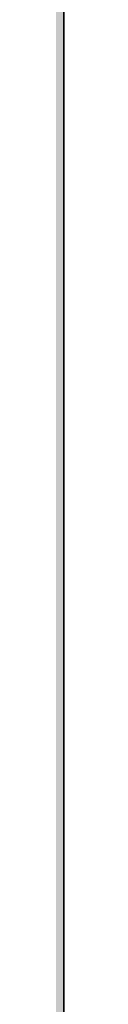
# Model space of a CAD drawing. Units: inches. Extents: x 2091 to 2899, y 967 to 2217.
# Tile 71 of 256: x 2212.144 to 2212.144, y 1102.499 to 1105.165. Entities that reach past the tile are written whole.
import ezdxf

# ---------------------------------------------------------------- set-up
doc = ezdxf.new("R2010")
doc.units = ezdxf.units.IN
doc.layers.add('A-WALL', color=7, linetype='Continuous', lineweight=35)
doc.layers.add('A-WALL-PATT', color=141, linetype='Continuous', lineweight=13, true_color=0xadddf7)

msp = doc.modelspace()

# ---------------------------------------------------------------- hatches: boundary and pattern name
at = {"layer": 'A-WALL-PATT'}
h = msp.add_hatch(color=256, dxfattribs=at)
h.dxf.hatch_style = 1
h.paths.add_polyline_path([(2212.1436, 1941.4191), (2387.6436, 1941.4191), (2387.6436, 1824.4191), (2392.1436, 1824.4191), (2392.1436, 1941.4191), (2609.6436, 1941.4191), (2609.6436, 1825.9191), (2614.1436, 1825.9191), (2614.1436, 1941.4191), (2794.1436, 1941.4191), (2794.1436, 1928.7622), (2803.1436, 1928.7622), (2803.1436, 2050.9191), (2203.1436, 2050.9191), (2203.1436, 1900.7579), (2212.1436, 1900.7579)])
h.paths.add_polyline_path([(2212.1436, 1945.9191), (2212.1436, 2041.9191), (2794.1436, 2041.9191), (2794.1436, 1945.9191), (2402.2482, 1945.9191), (2401.1024, 1945.7758), (2398.7024, 1945.7758)], flags=16)
h.paths.add_polyline_path([(2230.2299, 1948.0628), (2227.3499, 1949.5028), (2225.9099, 1951.9028), (2223.9899, 1952.8628), (2223.0299, 1955.2628), (2222.0699, 1959.5828), (2222.0699, 1963.4228), (2223.0299, 1965.6628), (2223.9899, 1965.3428), (2225.5859, 1963.8607), (2226.9115, 1964.9573), (2226.9489, 1965.9388), (2227.7783, 1966.9521), (2228.1999, 1968.8787), (2230.7099, 1964.8628), (2233.5899, 1966.3028), (2233.6073, 1966.3319), (2233.7727, 1964.9382), (2234.6338, 1963.6765), (2235.0299, 1963.9028), (2236.282, 1965.5724), (2235.9899, 1962.9428), (2237.9545, 1957.54), (2238.3899, 1957.9028), (2239.2159, 1960.3058), (2238.6546, 1966.385), (2238.6928, 1966.4381), (2238.8406, 1967.4997), (2238.7803, 1967.6875), (2238.8805, 1967.7868), (2238.6669, 1966.2518), (2239.2159, 1960.3058), (2238.3899, 1957.9028), (2236.9499, 1956.7028), (2234.5499, 1949.9828)], flags=0)
h.paths.add_polyline_path([(2278.012, 1948.0628), (2276.4964, 1947.8733), (2275.8498, 1947.6886), (2274.652, 1947.1028)], flags=0)
h.paths.add_polyline_path([(2269.852, 1955.7428), (2268.2762, 1956.6293), (2270.8673, 1956.3484), (2269.372, 1958.1428), (2268.715, 1959.1923), (2270.5698, 1958.7286), (2268.5807, 1961.9061), (2270.812, 1960.8919), (2270.812, 1963.4228), (2271.3933, 1964.7793), (2270.2918, 1966.1562), (2271.772, 1965.6628), (2272.1414, 1966.5248), (2273.9298, 1965.9286), (2275.6304, 1968.0543), (2276.3319, 1966.7219), (2276.5204, 1966.9521), (2276.942, 1968.8787), (2277.7343, 1967.6111), (2278.1399, 1969.4645), (2279.6591, 1967.0337), (2280.412, 1966.7828), (2280.9493, 1967.5888), (2281.6098, 1967.3686), (2282.1333, 1968.1538), (2282.3492, 1966.3334), (2282.3498, 1966.3326), (2283.4076, 1968.0954), (2283.7126, 1965.524), (2284.3202, 1964.6338), (2284.5118, 1964.8892), (2284.235, 1965.7048), (2284.5005, 1967.319), (2284.9079, 1965.4174), (2285.3963, 1966.0686), (2285.4328, 1966.2906), (2285.4733, 1966.1713), (2286.3539, 1967.3454), (2286.222, 1966.1582), (2287.6635, 1968.0802), (2287.714, 1968.4428), (2288.4816, 1969.0167), (2288.574, 1968.7289), (2288.9175, 1969.069), (2288.6068, 1966.8376), (2288.9287, 1963.3513), (2288.935, 1963.3568), (2288.9297, 1963.3404), (2289.0153, 1962.4139), (2290.1112, 1963.8751), (2290.1328, 1963.9426), (2290.2177, 1964.0171), (2290.1112, 1963.8751), (2289.1558, 1960.8916), (2288.594, 1959.2572), (2288.572, 1959.1028), (2289.532, 1960.5428), (2290.012, 1962.4628), (2290.1918, 1962.6427), (2289.7698, 1959.6886), (2286.8898, 1957.2886), (2284.4898, 1950.5686), (2283.3147, 1950.0463), (2283.292, 1949.9828), (2280.2901, 1948.6486), (2281.1298, 1948.6486), (2282.5698, 1948.1686), (2283.2047, 1948.0628), (2278.972, 1948.0628), (2276.092, 1949.5028), (2274.652, 1951.9028), (2272.732, 1952.8628)], flags=0)
h.paths.add_polyline_path([(2271.1589, 1958.0218), (2272.9698, 1955.8486), (2272.0098, 1960.1686), (2272.0098, 1964.0086), (2272.6244, 1965.4427), (2274.328, 1963.8607), (2275.6536, 1964.9573), (2275.6377, 1964.5391), (2277.4122, 1966.0069), (2277.033, 1965.1568), (2276.8299, 1964.9756), (2276.766, 1963.295), (2277.4496, 1962.6602), (2279.452, 1964.8628), (2282.332, 1966.3028), (2283.5298, 1966.8886), (2283.2945, 1966.7709), (2283.913, 1963.8847), (2284.8992, 1964.4483), (2284.732, 1962.9428), (2286.6966, 1957.54), (2287.132, 1957.9028), (2287.5419, 1959.0954), (2287.7794, 1958.4423), (2285.6827, 1956.6951), (2285.8765, 1959.7953), (2284.732, 1962.9428), (2284.8992, 1964.4483), (2283.913, 1963.8847), (2284.2238, 1962.4341), (2283.4244, 1963.6055), (2281.6098, 1962.5686), (2281.1298, 1960.1686), (2282.0898, 1956.3286), (2283.0498, 1952.9686), (2282.5698, 1950.5686), (2280.1698, 1948.6486), (2279.8833, 1948.7919), (2278.972, 1948.0628), (2278.972, 1949.0228), (2278.6723, 1949.3974), (2277.2898, 1950.0886), (2275.8498, 1952.4886), (2273.9298, 1953.4486), (2272.4898, 1954.8886), (2271.9216, 1954.8886), (2271.772, 1955.2628)], flags=0)
h.paths.add_polyline_path([(2311.9941, 1955.7428), (2312.0627, 1955.6742), (2312.0551, 1955.7085)], flags=0)
h.paths.add_polyline_path([(2331.9561, 1963.9518), (2333.3961, 1965.3918), (2331.0771, 1963.3568), (2330.9986, 1963.1115)], flags=0)
h.paths.add_polyline_path([(2310.5541, 1954.3028), (2307.0398, 1956.2799), (2310.7629, 1955.8763), (2312.4741, 1953.8228), (2313.4341, 1951.4228), (2315.3541, 1950.4628), (2316.7941, 1948.0628), (2317.4661, 1947.7268), (2319.3687, 1947.9646), (2317.7541, 1949.9828), (2317.5695, 1950.6105), (2316.7941, 1951.9028), (2314.8741, 1952.8628), (2313.9141, 1955.2628), (2311.5141, 1958.1428), (2309.3755, 1961.5592), (2311.5141, 1960.3371), (2311.5141, 1961.9828), (2310.6047, 1963.1196), (2311.7266, 1962.4785), (2312.4183, 1964.0926), (2312.256, 1964.2955), (2313.1941, 1963.9828), (2313.9141, 1965.6628), (2314.6468, 1965.4186), (2315.3541, 1966.3028), (2316.7941, 1967.7428), (2316.1574, 1966.9469), (2317.0341, 1965.2819), (2317.2226, 1965.5121), (2317.777, 1968.0458), (2318.4741, 1966.7219), (2318.6626, 1966.9521), (2319.0842, 1968.8787), (2321.207, 1965.4821), (2322.1614, 1966.9137), (2322.5541, 1966.7828), (2322.786, 1967.1306), (2322.8816, 1966.3243), (2323.312, 1965.7217), (2323.6513, 1965.8914), (2324.3965, 1967.1334), (2324.6569, 1964.9382), (2324.972, 1964.4766), (2325.3873, 1967.0015), (2325.9408, 1964.4183), (2327.2289, 1966.1358), (2327.1663, 1965.5724), (2328.0591, 1966.7628), (2328.2246, 1966.2475), (2329.668, 1967.6769), (2329.6646, 1967.6875), (2329.7648, 1967.7868), (2329.5511, 1966.2518), (2330.1001, 1960.3058), (2329.3328, 1958.0735), (2329.3131, 1957.9352), (2329.6341, 1958.2028), (2330.2341, 1959.1028), (2330.7141, 1961.0228), (2331.0341, 1961.3428), (2330.7141, 1959.1028), (2329.6341, 1958.2028), (2329.2741, 1957.6628), (2327.7121, 1956.3611), (2325.4341, 1949.9828), (2324.3338, 1949.4937), (2323.9941, 1948.5428), (2319.6741, 1946.6228), (2316.7941, 1948.0628), (2315.3541, 1950.4628), (2313.4341, 1951.4228)], flags=0)
h.paths.add_polyline_path([(2321.3357, 1947.952), (2321.1141, 1948.0628), (2321.1141, 1949.0228), (2319.1941, 1951.4228), (2316.7941, 1959.5828), (2316.6632, 1959.5828), (2315.3541, 1958.1428), (2314.3941, 1958.1428), (2313.1483, 1958.7091), (2312.9541, 1959.5828), (2312.9541, 1960.8919), (2315.8341, 1959.5828), (2316.6632, 1959.5828), (2317.3147, 1960.2994), (2315.0302, 1962.4207), (2316.3558, 1963.5173), (2316.3723, 1963.9516), (2316.4702, 1963.8607), (2317.7958, 1964.9573), (2317.7552, 1963.8897), (2319.1751, 1965.1568), (2319.4984, 1965.8814), (2321.1141, 1965.3428), (2323.2359, 1962.3724), (2325.6863, 1963.7726), (2325.5428, 1962.4806), (2325.1988, 1963.494), (2324.4785, 1963.0824), (2324.926, 1960.9941), (2324.0781, 1962.2365), (2322.4148, 1961.286), (2322.0741, 1959.5828), (2323.0341, 1955.7428), (2323.9941, 1952.3828), (2323.5141, 1949.9828), (2322.1427, 1948.8856), (2322.0741, 1948.5428)], flags=0)
h.paths.add_polyline_path([(2320.2075, 1963.3375), (2320.1541, 1963.4228), (2320.3941, 1963.5428)], flags=0)
h.paths.add_polyline_path([(2353.8505, 1965.8105), (2354.0305, 1965.7505), (2354.3305, 1966.4505), (2354.3305, 1966.9305)], flags=0)
h.paths.add_polyline_path([(2359.0206, 1969.0264), (2359.0984, 1968.9019), (2359.2335, 1969.5195), (2359.2335, 1969.9995)], flags=0)
h.paths.add_polyline_path([(2358.2567, 1966.6817), (2357.9836, 1966.348), (2358.2113, 1966.1462), (2358.4105, 1966.3896)], flags=0)
h.paths.add_polyline_path([(2357.7685, 1966.0588), (2357.7322, 1965.105), (2357.751, 1965.1206), (2357.7695, 1965.6065), (2357.7695, 1966.0578)], flags=0)
h.paths.add_polyline_path([(2359.1115, 1965.3045), (2359.1115, 1964.8245), (2359.8445, 1966.4675), (2359.8445, 1966.9475)], flags=0)
h.paths.add_polyline_path([(2360.2237, 1966.6214), (2360.6985, 1969.3625), (2360.6985, 1969.8425), (2360.2105, 1967.0255), (2360.2105, 1966.6425)], flags=0)
h.paths.add_polyline_path([(2363.4505, 1967.8905), (2363.4505, 1968.3705), (2362.4905, 1966.9305), (2362.656, 1966.6988)], flags=0)
h.paths.add_polyline_path([(2364.4755, 1966.0788), (2365.8505, 1968.3705), (2365.8505, 1968.8505), (2364.428, 1966.4796)], flags=0)
h.paths.add_polyline_path([(2366.3135, 1965.8525), (2366.3667, 1965.6958), (2366.8025, 1968.3455), (2366.8025, 1968.8255)], flags=0)
h.paths.add_polyline_path([(2367.1653, 1965.8035), (2367.2905, 1966.9305), (2367.2905, 1967.4105), (2367.1027, 1965.7201)], flags=0)
h.paths.add_polyline_path([(2370.0365, 1959.9735), (2371.0135, 1963.0245), (2371.0135, 1963.5045), (2370.0365, 1960.4535)], flags=0)
h.paths.add_polyline_path([(2371.6105, 1960.2105), (2372.5705, 1961.6505), (2372.5705, 1962.1305), (2371.8025, 1960.9785)], flags=0)
h.paths.add_polyline_path([(2350.8737, 1956.0051), (2351.9305, 1955.8905), (2354.4905, 1953.3305), (2353.8505, 1954.9305), (2351.4505, 1957.8105), (2347.9355, 1963.4255), (2347.9355, 1963.9055), (2351.4505, 1958.2905), (2353.7051, 1955.585), (2352.8905, 1959.2505), (2352.8905, 1959.7305), (2352.8905, 1961.9248), (2356.7305, 1959.7305), (2358.4545, 1961.6268), (2354.8105, 1965.0105), (2355.0309, 1965.2859), (2358.6911, 1961.8871), (2361.5305, 1965.0105), (2364.3765, 1966.4335), (2364.5244, 1965.1869), (2365.4545, 1963.8242), (2365.8811, 1964.068), (2365.3705, 1966.4505), (2365.3705, 1966.9305), (2366.8105, 1960.2105), (2366.8105, 1959.7305), (2366.3887, 1952.9814), (2367.7705, 1956.8505), (2368.6412, 1957.5761), (2366.8105, 1962.6105), (2366.8105, 1963.0905), (2368.7752, 1957.6877), (2369.2105, 1958.0505), (2370.0016, 1960.3519), (2369.4752, 1966.0527), (2369.5135, 1966.1058), (2369.5142, 1966.1109), (2369.4752, 1966.5327), (2369.5135, 1966.5858), (2369.6146, 1967.3126), (2369.1825, 1968.6585), (2369.1825, 1969.1385), (2369.601, 1967.8352), (2369.7012, 1967.9345), (2369.7179, 1968.0547), (2370.1452, 1968.3741), (2369.7787, 1968.0112), (2369.7012, 1967.4545), (2370.4682, 1968.214), (2369.6749, 1967.2658), (2369.5142, 1966.1109), (2370.0365, 1960.4535), (2370.0365, 1959.9735), (2369.4418, 1958.2432), (2370.6505, 1959.2505), (2371.0458, 1962.0176), (2371.1305, 1962.1305), (2370.6505, 1958.7705), (2367.7705, 1956.3705), (2365.3705, 1949.6505), (2362.0791, 1948.1876), (2363.4505, 1947.7305), (2361.0505, 1947.7305), (2360.0905, 1947.7305), (2357.1039, 1947.3572), (2360.0905, 1948.2105), (2358.1705, 1949.1705), (2356.7305, 1951.5705), (2354.8105, 1952.5305), (2351.9305, 1955.4105)], flags=0)
h.paths.add_polyline_path([(2361.0505, 1948.6905), (2359.1305, 1951.0905), (2356.7305, 1959.2505), (2355.7705, 1959.2505), (2352.8905, 1960.5596), (2352.8905, 1961.4448), (2355.8905, 1959.7305), (2356.7305, 1959.7305), (2356.8372, 1959.3678), (2361.5305, 1964.5305), (2363.2484, 1965.3894), (2364.9253, 1963.0418), (2362.4905, 1961.6505), (2362.0639, 1959.5172), (2362.9705, 1955.8905), (2363.9305, 1952.5305), (2363.9305, 1952.0505), (2363.4505, 1949.6505), (2361.0505, 1947.7305)], flags=0)
h.paths.add_polyline_path([(2359.1305, 1951.5705), (2359.2905, 1951.3705), (2361.0505, 1954.4505), (2361.0505, 1954.9305)], flags=0)
h.paths.add_polyline_path([(2357.2195, 1966.5455), (2356.7925, 1968.8145), (2356.7925, 1969.2945), (2357.2195, 1967.0255)], flags=0)
h.paths.add_polyline_path([(2361.0505, 1954.4505), (2361.5305, 1958.7705), (2361.5305, 1959.2505), (2361.0505, 1954.9305)], flags=0)
h.paths.add_polyline_path([(2402.5483, 1948.4861), (2402.3024, 1948.4158), (2402.5904, 1948.4158)], flags=0)
h.paths.add_polyline_path([(2394.1424, 1956.0958), (2395.6851, 1954.5532), (2396.7205, 1953.9707), (2396.0624, 1955.6158), (2395.2414, 1956.6011), (2395.8789, 1956.4417), (2395.1024, 1959.9358), (2395.1024, 1963.7758), (2396.0624, 1966.0158), (2397.0224, 1965.6958), (2398.6185, 1964.2138), (2399.9441, 1965.3103), (2399.9814, 1966.2918), (2400.8109, 1967.3052), (2401.2325, 1969.2317), (2403.5379, 1965.543), (2403.942, 1967.3893), (2404.7024, 1967.1358), (2405.4603, 1966.0748), (2406.6224, 1966.6558), (2406.6399, 1966.6849), (2406.8052, 1965.2912), (2406.9257, 1965.1147), (2407.3424, 1964.9758), (2407.8743, 1965.7737), (2408.1691, 1964.3981), (2409.3146, 1965.9254), (2409.2175, 1965.0511), (2409.4452, 1963.1312), (2410.3064, 1961.8695), (2410.7024, 1962.0958), (2411.4423, 1963.0823), (2411.1654, 1963.8978), (2411.6164, 1966.6398), (2411.7254, 1966.7911), (2411.8732, 1967.8527), (2411.8129, 1968.0405), (2411.9131, 1968.1398), (2411.6994, 1966.6048), (2412.2484, 1960.6588), (2413.2254, 1963.7098), (2414.3779, 1964.7212), (2414.5132, 1965.6927), (2414.4529, 1965.8805), (2414.5531, 1965.9798), (2414.3779, 1964.7212), (2414.5198, 1964.8457), (2414.3654, 1964.6311), (2414.3394, 1964.4448), (2414.8884, 1958.4988), (2414.0624, 1956.0958), (2412.6224, 1954.8958), (2410.1714, 1948.0329), (2410.0167, 1948.0844), (2405.9024, 1946.2558), (2405.9024, 1947.2158), (2405.2043, 1948.0886), (2404.2224, 1948.4158), (2403.2624, 1948.4158), (2400.3824, 1949.8558), (2399.6624, 1951.0558), (2397.9824, 1952.7358), (2397.0224, 1953.2158), (2395.6851, 1954.5532), (2392.6568, 1956.2569)], flags=0)
h.paths.add_polyline_path([(2409.0857, 1964.4074), (2409.1304, 1964.2757), (2409.2624, 1964.4958)], flags=0)
h.paths.add_polyline_path([(2397.7424, 1961.6158), (2398.7024, 1963.8558), (2399.6624, 1963.5358), (2401.4266, 1965.741), (2401.7914, 1966.5588), (2402.0714, 1965.0708), (2402.8355, 1964.3934), (2403.2624, 1964.9149), (2403.3381, 1964.7711), (2402.6155, 1963.9762), (2402.4986, 1960.9022), (2403.543, 1959.9325), (2404.4132, 1960.8897), (2404.7024, 1962.3358), (2407.9163, 1964.1724), (2409.5202, 1961.9269), (2410.9871, 1957.893), (2411.4224, 1958.2558), (2412.048, 1960.0756), (2412.4103, 1959.0791), (2411.6756, 1958.4668), (2411.6624, 1958.2558), (2411.6261, 1958.4255), (2409.9824, 1957.0558), (2407.5824, 1950.3358), (2403.2624, 1948.4158), (2403.2624, 1949.3758), (2401.3424, 1951.7758), (2399.4165, 1958.324), (2397.7424, 1959.0849), (2397.7424, 1959.9701), (2397.1024, 1960.3358), (2397.7424, 1960.0449)], flags=0)
h.paths.add_polyline_path([(2405.9024, 1952.9758), (2405.9504, 1953.4078), (2406.0167, 1953.1758)], flags=0)
h.paths.add_polyline_path([(2449.8178, 1967.114), (2449.7523, 1967.1358), (2449.7937, 1967.0779)], flags=0)
h.paths.add_polyline_path([(2451.6977, 1966.6181), (2451.7409, 1966.6901), (2451.6921, 1966.6657)], flags=0)
h.paths.add_polyline_path([(2454.3436, 1965.7376), (2455.7523, 1967.6158), (2455.9923, 1968.0958), (2454.3645, 1965.9254)], flags=0)
h.paths.add_polyline_path([(2457.5473, 1968.8638), (2457.7873, 1969.3438), (2457.0543, 1968.7958), (2457.0076, 1968.4603)], flags=0)
h.paths.add_polyline_path([(2456.9218, 1967.8567), (2456.8022, 1968.229), (2456.723, 1967.6598)], flags=0)
h.paths.add_polyline_path([(2457.3023, 1967.3768), (2457.5423, 1967.8568), (2456.8103, 1966.8398), (2456.7405, 1966.7002), (2456.749, 1966.6081)], flags=0)
h.paths.add_polyline_path([(2458.2753, 1963.7098), (2458.1553, 1963.3352), (2460.3543, 1965.2648), (2460.5943, 1965.7448)], flags=0)
h.paths.add_polyline_path([(2458.3923, 1962.8158), (2458.3641, 1962.6182), (2459.5923, 1964.2558), (2459.8323, 1964.7358)], flags=0)
h.paths.add_polyline_path([(2459.3523, 1962.8158), (2459.2723, 1962.4958), (2460.0723, 1963.2958), (2460.3123, 1963.7758)], flags=0)
h.paths.add_polyline_path([(2458.6803, 1960.6078), (2458.6323, 1960.4158), (2459.5923, 1961.8558), (2459.8323, 1962.3358)], flags=0)
h.paths.add_polyline_path([(2437.8382, 1956.2427), (2439.1923, 1956.0958), (2441.3523, 1953.9358), (2440.8723, 1955.1358), (2438.4723, 1958.0158), (2438.0716, 1958.656), (2438.7123, 1958.4958), (2440.6396, 1956.1831), (2439.9123, 1959.4558), (2439.9123, 1963.2958), (2441.3523, 1966.6558), (2441.5923, 1967.1358), (2441.1123, 1966.0158), (2442.0723, 1965.6958), (2443.989, 1968.0917), (2444.2413, 1966.7508), (2444.9168, 1966.1519), (2445.6766, 1967.0801), (2446.2553, 1969.7248), (2446.4953, 1970.2048), (2446.2824, 1969.2317), (2447.3627, 1967.5033), (2447.7203, 1969.5678), (2447.9603, 1970.0478), (2447.4855, 1967.3068), (2448.7923, 1965.2158), (2448.4723, 1964.8638), (2448.5523, 1964.7358), (2451.4521, 1966.1857), (2451.6151, 1964.8112), (2452.3079, 1963.7962), (2453.2345, 1964.3257), (2454.0723, 1960.4158), (2453.6287, 1953.3177), (2454.7923, 1956.5758), (2455.0323, 1957.0558), (2455.7188, 1957.6279), (2453.8323, 1962.8158), (2453.941, 1963.7936), (2453.3353, 1965.5778), (2453.8243, 1968.5508), (2454.0643, 1969.0308), (2453.5753, 1966.0578), (2454.0403, 1964.6879), (2453.8323, 1962.8158), (2455.7188, 1957.6279), (2456.3672, 1958.1682), (2457.0583, 1960.1788), (2457.2983, 1960.6588), (2456.4723, 1958.2558), (2457.7177, 1959.2937), (2457.6723, 1958.9758), (2454.89, 1956.6572), (2453.6141, 1953.0849), (2453.5923, 1952.7358), (2453.3523, 1952.2558), (2453.3596, 1952.3722), (2452.6323, 1950.3358), (2452.3923, 1949.8558), (2449.2038, 1948.4387), (2450.7123, 1947.9358), (2448.0723, 1947.9358), (2447.1123, 1947.9358), (2444.5523, 1947.6158), (2447.1996, 1948.3722), (2445.1923, 1949.3758), (2443.7523, 1951.7758), (2441.8323, 1952.7358), (2438.9523, 1955.6158)], flags=0)
h.paths.add_polyline_path([(2443.9923, 1959.9358), (2444.0403, 1959.7726), (2444.1216, 1959.862)], flags=0)
h.paths.add_polyline_path([(2442.9123, 1959.9358), (2443.0323, 1959.9358), (2442.4457, 1960.2025)], flags=0)
h.paths.add_polyline_path([(2444.9829, 1965.0197), (2445.2793, 1965.2648), (2445.5193, 1965.7448), (2444.994, 1965.3103)], flags=0)
h.paths.add_polyline_path([(2446.1333, 1965.0298), (2446.3304, 1965.4715), (2444.9703, 1964.2578), (2444.7303, 1963.7778)], flags=0)
h.paths.add_polyline_path([(2442.7923, 1959.4558), (2443.7523, 1959.4558), (2446.1523, 1951.2958), (2446.4123, 1951.7508), (2446.3923, 1951.7758), (2448.0806, 1954.7303), (2448.5523, 1958.9758), (2441.8323, 1965.2158), (2442.1549, 1965.6191), (2448.7923, 1959.4558), (2448.3123, 1955.1358), (2448.0723, 1954.6558), (2446.4123, 1951.7508), (2448.3123, 1949.3758), (2448.3123, 1948.4158), (2450.5409, 1950.1987), (2450.9523, 1952.2558), (2449.9923, 1955.6158), (2449.0323, 1959.4558), (2449.5123, 1961.8558), (2449.7523, 1962.3358), (2449.6749, 1961.9487), (2452.9945, 1963.8457), (2453.0644, 1963.5194), (2452.8846, 1963.7829), (2449.6749, 1961.9487), (2449.2723, 1959.9358), (2450.2323, 1956.0958), (2451.1923, 1952.7358), (2450.7123, 1950.3358), (2450.4723, 1949.8558), (2448.0723, 1947.9358), (2448.0723, 1948.5358), (2445.4323, 1949.8558), (2443.9923, 1952.2558), (2442.0723, 1953.2158), (2441.1123, 1955.6158), (2440.1523, 1959.9358), (2440.1523, 1960.6558)], flags=0)
h.paths.add_polyline_path([(2456.6923, 1966.9858), (2457.6083, 1968.0808), (2457.8483, 1968.5608), (2456.9323, 1967.4658)], flags=0)
h.paths.add_polyline_path([(2489.8966, 1966.5802), (2489.9429, 1966.1893), (2490.7475, 1967.5302), (2491.3191, 1968.9512)], flags=0)
h.paths.add_polyline_path([(2473.5625, 1956.4071), (2477.14, 1956.0193), (2476.9553, 1956.2408), (2475.108, 1957.2801), (2476.3475, 1956.9702), (2475.1869, 1958.8242), (2476.9191, 1958.3912), (2475.4116, 1960.7993), (2477.7875, 1959.7193), (2477.7875, 1962.2502), (2477.6374, 1962.4379), (2477.8226, 1962.3321), (2478.3591, 1963.5841), (2478.3591, 1963.6712), (2477.3243, 1964.9646), (2478.7148, 1964.5011), (2479.3191, 1965.9112), (2480.2791, 1965.5912), (2481.784, 1967.4722), (2482.1165, 1965.7052), (2482.8806, 1965.0278), (2483.2093, 1965.4294), (2483.2202, 1965.7151), (2483.0759, 1965.989), (2483.7118, 1966.7658), (2484.1305, 1968.6792), (2484.7021, 1970.1002), (2484.4892, 1969.1271), (2486.5029, 1965.9051), (2487.3875, 1965.6102), (2488.1534, 1966.7591), (2488.717, 1965.9701), (2489.2001, 1966.2116), (2489.3307, 1965.111), (2490.3939, 1963.6225), (2490.6608, 1963.775), (2490.4939, 1964.5536), (2490.9231, 1963.9248), (2491.3191, 1964.1512), (2491.3334, 1964.1702), (2491.2105, 1964.5322), (2491.2818, 1964.9655), (2491.4258, 1964.2934), (2494.0765, 1967.8276), (2494.4979, 1966.5149), (2494.5982, 1966.6142), (2494.6895, 1967.2702), (2495.1067, 1967.5822), (2495.1298, 1967.7481), (2495.0696, 1967.9359), (2495.1698, 1968.0351), (2495.0318, 1967.0436), (2495.7538, 1967.7587), (2494.9821, 1966.6864), (2494.9561, 1966.5002), (2495.479, 1960.8369), (2495.9105, 1962.1842), (2496.4821, 1963.6052), (2496.0727, 1962.3266), (2496.7689, 1962.9375), (2496.5991, 1962.7112), (2496.1191, 1959.3512), (2496.7329, 1960.2718), (2496.9875, 1961.2902), (2497.5591, 1962.7112), (2497.0791, 1960.7912), (2496.5075, 1959.3702), (2495.5475, 1957.9302), (2492.7588, 1955.6064), (2490.8391, 1950.2312), (2490.2675, 1948.8102), (2485.9475, 1946.8902), (2483.0675, 1948.3302), (2481.6275, 1950.7302), (2479.7075, 1951.6902), (2476.8275, 1954.5702)], flags=0)
h.paths.add_polyline_path([(2485.577, 1948.3134), (2485.5591, 1948.3112), (2485.5788, 1948.3112)], flags=0)
h.paths.add_polyline_path([(2478.6451, 1954.5512), (2478.109, 1956.9633), (2479.3191, 1955.5112), (2480.2791, 1953.1112), (2482.1991, 1952.1512), (2483.6391, 1949.7512), (2486.5191, 1948.3112), (2486.5191, 1949.2712), (2484.7393, 1951.4959), (2484.0275, 1950.2502), (2481.6275, 1958.4102), (2482.3751, 1959.2327), (2482.1991, 1959.8312), (2483.1976, 1960.9295), (2479.7075, 1964.1702), (2480.6034, 1965.2901), (2481.8752, 1964.1091), (2482.6664, 1964.7636), (2482.6154, 1963.4218), (2482.9892, 1963.0747), (2484.0085, 1963.9842), (2484.6836, 1965.4975), (2484.5801, 1965.4052), (2485.3573, 1967.1471), (2485.1206, 1965.7812), (2486.4275, 1963.6902), (2488.1454, 1964.5492), (2489.8223, 1962.2016), (2490.7475, 1962.7302), (2491.9997, 1964.3998), (2492.076, 1965.0873), (2492.2129, 1964.6841), (2492.4854, 1965.0474), (2492.2791, 1963.1912), (2494.2438, 1957.7884), (2494.5625, 1958.054), (2494.9335, 1959.1332), (2495.5051, 1960.5542), (2494.6791, 1958.1512), (2494.1075, 1956.7302), (2494.5625, 1958.054), (2493.4085, 1957.0923), (2491.7075, 1961.7702), (2491.9997, 1964.3998), (2490.7475, 1962.7302), (2487.712, 1960.9957), (2487.4791, 1959.8312), (2488.4391, 1955.9912), (2489.3991, 1952.6312), (2488.9191, 1950.2312), (2488.5769, 1949.9574), (2488.3475, 1948.8102), (2487.6517, 1948.2536), (2487.4791, 1948.3112), (2486.5191, 1948.3112), (2483.6391, 1949.7512), (2482.1991, 1952.1512), (2480.2791, 1953.1112), (2478.8391, 1954.5512)], flags=0)
h.paths.add_polyline_path([(2526.6483, 1966.9875), (2526.5173, 1967.0312), (2526.6001, 1966.9153)], flags=0)
h.paths.add_polyline_path([(2528.4706, 1966.4467), (2528.5745, 1966.6197), (2528.4571, 1966.561)], flags=0)
h.paths.add_polyline_path([(2534.1333, 1967.4962), (2534.1567, 1967.5428), (2534.0598, 1967.4083)], flags=0)
h.paths.add_polyline_path([(2536.1619, 1964.0506), (2535.1573, 1962.7112), (2535.1009, 1962.3159), (2536.1173, 1963.6712), (2536.4205, 1964.2775)], flags=0)
h.paths.add_polyline_path([(2535.1573, 1959.8312), (2536.1173, 1961.2712), (2536.5973, 1962.2312), (2535.2533, 1960.2152)], flags=0)
h.paths.add_polyline_path([(2513.249, 1956.2848), (2516.2212, 1955.9626), (2514.9973, 1957.4312), (2514.1958, 1958.7115), (2515.4773, 1958.3912), (2516.9319, 1956.6457), (2516.4373, 1958.8712), (2516.4373, 1962.7112), (2516.8727, 1963.727), (2515.3464, 1965.6348), (2517.3973, 1964.9512), (2517.8773, 1966.0712), (2518.3573, 1967.0312), (2517.8773, 1965.9112), (2518.8373, 1965.5912), (2520.4866, 1967.6527), (2520.7663, 1966.1662), (2521.5304, 1965.4887), (2521.7814, 1965.7954), (2521.8009, 1966.3073), (2521.4778, 1966.9209), (2521.2463, 1967.1262), (2521.1777, 1967.4909), (2521.4778, 1966.9209), (2522.0104, 1966.4487), (2522.2574, 1966.7504), (2522.7803, 1969.1402), (2523.2603, 1970.1002), (2523.0474, 1969.1271), (2524.6731, 1966.5259), (2526.0373, 1966.0712), (2526.7952, 1965.0101), (2527.9771, 1965.601), (2528.1401, 1964.2266), (2528.6646, 1963.4582), (2529.3886, 1963.8719), (2529.3297, 1964.147), (2529.4813, 1963.9248), (2529.8773, 1964.1512), (2529.984, 1964.2934), (2529.7891, 1965.2032), (2530.0624, 1964.3979), (2532.8025, 1968.0513), (2533.1478, 1966.9759), (2533.248, 1967.0751), (2533.3393, 1967.7312), (2533.6728, 1967.9805), (2533.728, 1968.0351), (2533.5143, 1966.5002), (2534.0247, 1960.9725), (2534.5603, 1962.6452), (2535.0403, 1963.6052), (2534.0633, 1960.5542), (2533.2373, 1958.1512), (2534.2882, 1959.0268), (2534.1973, 1958.3912), (2531.5126, 1956.1539), (2529.3973, 1950.2312), (2528.9173, 1949.2712), (2526.4488, 1948.174), (2527.4773, 1947.8312), (2530.3573, 1947.3512), (2524.5973, 1947.3512), (2521.7173, 1948.7912), (2520.2773, 1951.1912), (2518.3573, 1952.1512), (2515.4773, 1955.0312)], flags=0)
h.paths.add_polyline_path([(2523.9348, 1967.1903), (2523.6195, 1966.4837), (2523.7705, 1966.2421)], flags=0)
h.paths.add_polyline_path([(2518.8373, 1953.1112), (2517.8773, 1955.5112), (2516.885, 1959.9768), (2516.9173, 1959.9621), (2516.9173, 1962.0254), (2520.7573, 1959.8312), (2522.0249, 1961.2255), (2518.3573, 1964.6312), (2519.0026, 1965.4377), (2520.4334, 1964.1091), (2521.3011, 1964.8269), (2521.2452, 1963.3553), (2525.6383, 1959.276), (2526.0373, 1961.2712), (2529.3973, 1963.1912), (2530.6495, 1964.8607), (2530.6647, 1964.9976), (2530.692, 1964.9173), (2531.0878, 1965.4451), (2530.946, 1964.1689), (2530.692, 1964.9173), (2529.3973, 1963.1912), (2526.3625, 1961.457), (2526.0373, 1959.8312), (2526.9973, 1955.9912), (2527.9573, 1952.6312), (2527.4773, 1950.2312), (2527.1345, 1949.9569), (2526.9739, 1949.1541), (2526.6973, 1949.0312), (2524.5973, 1947.3512), (2524.5973, 1948.3112), (2524.2773, 1948.7112), (2522.1973, 1949.7512), (2520.7573, 1952.1512)], flags=0)
h.paths.add_polyline_path([(2520.2773, 1958.8712), (2520.8533, 1959.5048), (2523.1573, 1951.6712), (2524.6139, 1954.2201), (2524.5973, 1954.0712), (2522.6773, 1950.7112)], flags=0)
h.paths.add_polyline_path([(2559.3709, 1966.3112), (2559.3984, 1966.3249), (2559.4019, 1966.3453)], flags=0)
h.paths.add_polyline_path([(2549.7709, 1957.1912), (2552.6509, 1954.3112), (2552.134, 1955.6035), (2550.6109, 1957.4312), (2547.0959, 1963.0462), (2545.7759, 1965.2062), (2549.2909, 1959.5912), (2551.6909, 1956.7112), (2550.7929, 1960.7521), (2550.7309, 1960.7803), (2550.7309, 1964.8712), (2551.6909, 1967.1112), (2552.6509, 1966.7912), (2554.247, 1965.3091), (2555.0343, 1965.9603), (2555.5817, 1966.6446), (2555.6099, 1967.3872), (2556.4394, 1968.4005), (2556.861, 1970.3271), (2559.3709, 1966.3112), (2560.6909, 1964.1512), (2562.4088, 1965.0101), (2561.6509, 1966.0712), (2560.3309, 1968.2312), (2561.7585, 1966.2325), (2562.3472, 1967.1156), (2562.4337, 1966.3866), (2563.1278, 1965.3696), (2563.5709, 1965.5912), (2563.5884, 1965.6202), (2563.3625, 1967.5235), (2563.7225, 1965.8438), (2565.06, 1968.073), (2564.7329, 1965.1287), (2565.1176, 1963.3334), (2567.4446, 1966.4361), (2567.3156, 1967.8333), (2567.3538, 1967.8864), (2567.5016, 1968.9481), (2567.4413, 1969.1359), (2567.5416, 1969.2351), (2567.3279, 1967.7002), (2567.8769, 1961.7542), (2568.7467, 1964.4703), (2568.6356, 1965.6733), (2568.6738, 1965.7264), (2568.8216, 1966.7881), (2568.7613, 1966.9759), (2568.8616, 1967.0751), (2568.6479, 1965.5402), (2568.7261, 1964.693), (2568.8539, 1964.8052), (2568.7467, 1964.4703), (2568.8172, 1963.7063), (2568.9709, 1963.9112), (2568.8661, 1963.1773), (2569.1969, 1959.5942), (2568.3709, 1957.1912), (2566.9309, 1955.9912), (2564.6203, 1949.5214), (2564.6509, 1949.5112), (2564.6166, 1949.5112), (2564.5309, 1949.2712), (2560.2109, 1947.3512), (2557.3309, 1948.7912), (2556.0452, 1950.934), (2556.0109, 1950.9512), (2555.8566, 1951.2083), (2553.9709, 1952.1512), (2551.0909, 1955.0312), (2546.6501, 1957.5295)], flags=0)
h.paths.add_polyline_path([(2567.0258, 1959.3302), (2567.035, 1959.3049), (2567.0509, 1959.3512)], flags=0)
h.paths.add_polyline_path([(2551.9683, 1962.5184), (2553.0109, 1964.9512), (2553.9709, 1964.6312), (2555.567, 1963.1491), (2556.8926, 1964.2456), (2556.9299, 1965.2272), (2557.144, 1965.4887), (2556.4201, 1966.1306), (2556.3914, 1966.105), (2556.3799, 1966.1662), (2556.4201, 1966.1306), (2556.9519, 1966.6052), (2557.0921, 1966.9195), (2557.5709, 1966.0102), (2557.7594, 1966.2405), (2557.4179, 1964.6802), (2556.8926, 1964.2456), (2556.8071, 1961.9976), (2560.6909, 1958.3912), (2560.6355, 1957.8927), (2560.8109, 1957.1912), (2561.7709, 1953.8312), (2561.2909, 1951.4312), (2559.1104, 1949.6868), (2559.1565, 1949.6292), (2563.0265, 1951.3492), (2562.6109, 1949.2712), (2560.2109, 1947.3512), (2560.2109, 1948.3112), (2559.2509, 1949.5112), (2558.8909, 1949.5112), (2558.8909, 1949.9612), (2558.2909, 1950.7112), (2558.0537, 1951.5177), (2556.9709, 1952.8712), (2555.0679, 1959.3415), (2552.0509, 1961.0654), (2552.0509, 1962.4712)], flags=0)
h.paths.add_polyline_path([(2588.33, 1958.3912), (2588.6102, 1958.111), (2588.5534, 1958.3669)], flags=0)
h.paths.add_polyline_path([(2594.7455, 1950.4931), (2593.9575, 1953.172), (2593.13, 1954.5512), (2591.21, 1955.5112), (2590.25, 1957.9112), (2588.309, 1960.2404), (2586.1773, 1961.2093), (2587.85, 1960.7912), (2587.2534, 1961.7442), (2588.4413, 1961.0654), (2588.4413, 1962.6555), (2588.4217, 1962.6653), (2588.4413, 1962.7112), (2586.914, 1964.6203), (2588.8771, 1963.728), (2589.29, 1964.6915), (2589.29, 1966.0712), (2590.25, 1968.3112), (2591.21, 1967.9912), (2592.8061, 1966.5091), (2594.1317, 1967.6056), (2594.169, 1968.5872), (2594.9985, 1969.6005), (2595.4201, 1971.5271), (2597.93, 1967.5112), (2600.81, 1968.9512), (2600.8275, 1968.9802), (2600.9928, 1967.5866), (2601.854, 1966.3248), (2602.1071, 1966.4695), (2602.2364, 1967.2551), (2602.3567, 1966.6934), (2603.5022, 1968.2207), (2603.21, 1965.5912), (2605.1747, 1960.1884), (2605.5069, 1960.4652), (2605.026, 1965.6733), (2605.0642, 1965.7264), (2605.212, 1966.7881), (2605.1517, 1966.9759), (2605.252, 1967.0751), (2605.3433, 1967.7312), (2605.9529, 1968.1869), (2605.8748, 1969.0333), (2605.913, 1969.0864), (2606.0608, 1970.1481), (2606.0005, 1970.3359), (2606.1007, 1970.4351), (2605.887, 1968.9002), (2606.436, 1962.9542), (2605.61, 1960.5512), (2605.997, 1960.8737), (2606.5643, 1962.6452), (2608.2415, 1964.1169), (2608.01, 1963.1912), (2607.05, 1961.7512), (2606.6315, 1961.4024), (2606.2013, 1958.3912), (2603.3213, 1955.9912), (2600.9213, 1949.2712), (2596.6013, 1947.3512), (2593.7213, 1948.7912), (2592.8573, 1950.2312), (2592.65, 1950.2312)], flags=0)
h.paths.add_polyline_path([(2596.6013, 1947.3512), (2596.6013, 1948.3112), (2594.6813, 1950.7112), (2596.155, 1953.29), (2595.53, 1954.0712), (2593.1992, 1961.996), (2592.6513, 1962.5047), (2591.7802, 1963.0025), (2593.283, 1964.2456), (2593.3203, 1965.2272), (2594.1498, 1966.2405), (2594.5714, 1968.1671), (2596.1827, 1965.589), (2596.9513, 1966.4345), (2598.0413, 1966.0712), (2598.7992, 1965.0101), (2599.9613, 1965.5912), (2599.9788, 1965.6202), (2600.1441, 1964.2266), (2601.0053, 1962.9648), (2601.4013, 1963.1912), (2602.6535, 1964.8607), (2602.3613, 1962.2312), (2603.7927, 1958.2947), (2601.9776, 1953.2124), (2601.9462, 1952.7095), (2599.4688, 1951.6084), (2599.0013, 1949.2712)], flags=0)
h.paths.add_polyline_path([(2597.5613, 1958.8712), (2597.671, 1959.4194), (2597.5951, 1958.7362)], flags=0)
h.paths.add_polyline_path([(2623.6663, 1961.2544), (2625.5192, 1960.7912), (2624.9655, 1961.6755), (2627.1992, 1960.6603), (2627.1992, 1961.1512), (2626.9592, 1962.2312), (2626.9592, 1963.4912), (2625.5823, 1965.2122), (2626.9592, 1964.4254), (2626.9592, 1965.8312), (2626.8692, 1965.8612), (2627.9192, 1968.3112), (2628.8792, 1967.9912), (2630.4752, 1966.5091), (2631.8008, 1967.6056), (2631.8382, 1968.5872), (2632.6676, 1969.6005), (2633.0892, 1971.5271), (2635.5992, 1967.5112), (2638.4792, 1968.9512), (2638.4966, 1968.9802), (2638.662, 1967.5866), (2639.1763, 1966.833), (2639.7802, 1967.8396), (2640.0258, 1966.6934), (2641.1713, 1968.2207), (2640.8792, 1965.5912), (2641.1143, 1964.9446), (2641.4113, 1965.3407), (2641.3081, 1964.4116), (2642.8438, 1960.1884), (2643.2792, 1960.5512), (2644.0847, 1962.8947), (2643.7839, 1966.1533), (2643.8068, 1966.1852), (2643.6007, 1968.4181), (2643.5228, 1968.6606), (2643.7299, 1970.1481), (2643.6696, 1970.3359), (2643.7698, 1970.4351), (2643.5562, 1968.9002), (2643.6007, 1968.4181), (2643.9096, 1967.4559), (2644.0098, 1967.5551), (2643.8117, 1966.1321), (2644.1052, 1962.9542), (2644.2388, 1961.3508), (2644.7192, 1961.7512), (2645.0329, 1962.2217), (2645.3222, 1963.1252), (2646.0764, 1963.787), (2645.0329, 1962.2217), (2644.3452, 1960.0742), (2643.5192, 1957.6712), (2642.0792, 1956.4712), (2639.7196, 1949.8644), (2639.8755, 1949.8384), (2635.3592, 1947.8312), (2632.4792, 1949.2712), (2631.0392, 1951.6712), (2629.1192, 1952.6312), (2628.1592, 1955.0312), (2625.7592, 1957.9112)], flags=0)
h.paths.add_polyline_path([(2627.8163, 1956.574), (2627.3737, 1958.5657), (2626.3763, 1959.7626), (2627.1992, 1959.3512), (2627.3737, 1958.5657), (2627.9192, 1957.9112), (2628.8792, 1955.5112), (2630.7992, 1954.5512), (2632.2392, 1952.1512), (2633.315, 1951.6132), (2631.0392, 1959.3512), (2631.4978, 1959.8557), (2630.7992, 1962.2312), (2631.4499, 1962.9469), (2630.7152, 1963.6291), (2632.0408, 1964.7256), (2632.0782, 1965.7072), (2632.2922, 1965.9687), (2631.7053, 1966.4891), (2633.1364, 1967.7661), (2633.3292, 1968.6471), (2634.6747, 1966.4943), (2635.2085, 1967.0814), (2636.7992, 1966.5512), (2637.6764, 1967.867), (2638.9939, 1966.0225), (2639.7053, 1966.429), (2641.1192, 1959.8312), (2640.9301, 1956.8057), (2639.4392, 1952.6312), (2638.2275, 1952.0926), (2637.7592, 1949.7512), (2635.3592, 1947.8312), (2635.3592, 1948.7912), (2633.4392, 1951.1912), (2633.315, 1951.6132), (2632.2392, 1952.1512), (2630.7992, 1954.5512), (2628.8792, 1955.5112)], flags=0)
h.paths.add_polyline_path([(2637.7592, 1953.8312), (2637.2792, 1955.5112), (2636.3192, 1959.3512), (2636.7992, 1961.7512), (2639.2339, 1963.1425), (2637.5571, 1965.4901), (2638.7389, 1966.081), (2638.902, 1964.7066), (2639.7631, 1963.4448), (2636.7992, 1961.7512), (2636.5325, 1960.4178), (2637.0392, 1958.3912), (2637.9992, 1955.0312)], flags=0)
h.paths.add_polyline_path([(2668.5674, 1951.4312), (2667.6074, 1953.8312), (2665.2074, 1956.7112), (2662.2939, 1961.3653), (2665.4474, 1959.5912), (2666.6474, 1958.3912), (2666.6474, 1959.9752), (2666.0583, 1960.6821), (2666.6474, 1960.3454), (2666.6474, 1961.9912), (2666.7001, 1962.1141), (2666.4074, 1963.4312), (2666.4074, 1967.2712), (2667.3674, 1969.5112), (2668.3274, 1969.1912), (2669.9235, 1967.7091), (2671.2491, 1968.8056), (2671.2864, 1969.7872), (2672.1159, 1970.8005), (2672.5375, 1972.7271), (2675.0474, 1968.7112), (2677.9274, 1970.1512), (2677.9449, 1970.1802), (2678.1102, 1968.7866), (2678.9713, 1967.5248), (2679.3674, 1967.7512), (2680.6196, 1969.4207), (2680.3274, 1966.7912), (2682.2921, 1961.3884), (2682.7274, 1961.7512), (2683.3583, 1963.5866), (2683.2321, 1964.9533), (2683.2703, 1965.0064), (2683.3932, 1965.8891), (2683.36, 1966.2492), (2683.3578, 1966.2559), (2683.3592, 1966.2572), (2682.9921, 1970.2333), (2683.0303, 1970.2864), (2683.1781, 1971.3481), (2683.1178, 1971.5359), (2683.2181, 1971.6351), (2683.0044, 1970.1002), (2683.3592, 1966.2572), (2683.4581, 1966.3551), (2683.3932, 1965.8891), (2683.4139, 1965.665), (2684.4238, 1966.8723), (2683.5534, 1964.1542), (2683.3583, 1963.5866), (2683.7934, 1958.8742), (2682.9674, 1956.4712), (2681.5274, 1955.2712), (2680.1092, 1951.3003), (2680.0849, 1950.9116), (2679.9768, 1950.9296), (2679.1274, 1948.5512), (2674.8074, 1946.6312), (2671.9274, 1948.0712), (2670.4874, 1950.4712)], flags=0)
h.paths.add_polyline_path([(2671.9357, 1953.227), (2671.6874, 1953.3512), (2670.2474, 1955.7512), (2668.3274, 1956.7112), (2667.3567, 1959.1378), (2669.5274, 1958.1512), (2670.4874, 1958.1512), (2671.4794, 1959.2424), (2670.6844, 1961.9454), (2668.8896, 1963.612), (2667.3074, 1964.3312), (2668.5674, 1963.9112), (2668.8309, 1964.2406), (2670.2474, 1963.4312), (2672.4221, 1965.8234), (2672.7775, 1967.4471), (2673.2341, 1966.7165), (2674.4119, 1968.0121), (2673.9806, 1965.5221), (2675.2874, 1963.4312), (2675.5541, 1963.5645), (2675.9324, 1965.4562), (2676.2474, 1965.3512), (2677.0053, 1964.2901), (2678.1674, 1964.8712), (2679.6074, 1967.2712), (2680.3274, 1963.9112), (2680.3066, 1963.5775), (2680.3472, 1963.4576), (2680.8596, 1964.1407), (2680.5674, 1961.5112), (2681.1036, 1960.0366), (2678.8874, 1953.8312), (2677.0925, 1953.0334), (2677.6874, 1950.9512), (2677.2074, 1948.5512), (2674.8074, 1946.6312), (2674.8074, 1947.5912), (2672.8874, 1949.9912)], flags=0)
h.paths.add_polyline_path([(2673.9846, 1951.9112), (2674.5674, 1952.9312), (2674.5674, 1951.9112), (2676.9674, 1953.8312), (2677.4474, 1956.2312), (2676.4874, 1959.5912), (2676.2474, 1960.5512), (2679.7296, 1962.541), (2680.0593, 1961.0025), (2679.2113, 1962.2448), (2676.2474, 1960.5512), (2676.4874, 1959.5912), (2677.4474, 1956.2312), (2676.9674, 1953.8312), (2674.5674, 1951.9112)], flags=0)
h.paths.add_polyline_path([(2707.4793, 1952.8147), (2706.5193, 1955.2147), (2705.5593, 1959.5347), (2705.5593, 1963.3747), (2706.5193, 1965.6147), (2707.4793, 1965.2947), (2709.0753, 1963.8126), (2710.401, 1964.9091), (2710.4383, 1965.8907), (2711.2677, 1966.904), (2711.6893, 1968.8306), (2714.1993, 1964.8147), (2717.0793, 1966.2547), (2717.0967, 1966.2837), (2717.2621, 1964.8901), (2718.1232, 1963.6283), (2718.5193, 1963.8547), (2719.7715, 1965.5242), (2719.4793, 1962.8947), (2721.4439, 1957.4919), (2721.8793, 1957.8547), (2722.7053, 1960.2577), (2722.144, 1966.3368), (2722.1822, 1966.3899), (2722.33, 1967.4516), (2722.2697, 1967.6393), (2722.37, 1967.7386), (2722.1563, 1966.2037), (2722.7053, 1960.2577), (2721.8793, 1957.8547), (2720.4393, 1956.6547), (2718.0393, 1949.9347), (2713.7193, 1948.0147), (2710.8393, 1949.4547), (2709.3993, 1951.8547)], flags=0)
h.paths.add_polyline_path([(2749.3012, 1952.8147), (2748.3412, 1955.2147), (2747.3812, 1959.5347), (2747.3812, 1963.3747), (2748.3412, 1965.6147), (2749.3012, 1965.2947), (2750.8973, 1963.8126), (2752.2229, 1964.9091), (2752.2602, 1965.8907), (2753.0897, 1966.904), (2753.5113, 1968.8306), (2756.0212, 1964.8147), (2758.9012, 1966.2547), (2758.9187, 1966.2837), (2759.084, 1964.8901), (2759.9452, 1963.6283), (2760.3412, 1963.8547), (2761.5934, 1965.5242), (2761.3012, 1962.8947), (2763.2659, 1957.4919), (2763.7012, 1957.8547), (2764.5272, 1960.2577), (2763.9659, 1966.3368), (2764.0042, 1966.3899), (2764.1519, 1967.4516), (2764.0917, 1967.6393), (2764.1919, 1967.7386), (2763.9782, 1966.2037), (2764.5272, 1960.2577), (2763.7012, 1957.8547), (2762.2612, 1956.6547), (2759.8612, 1949.9347), (2755.5412, 1948.0147), (2752.6612, 1949.4547), (2751.2212, 1951.8547)], flags=0)
h.paths.add_polyline_path([(2212.1436, 1819.9345), (2203.1436, 1819.9345), (2203.1436, 1739.9795), (2212.1436, 1739.9795), (2212.1436, 1780.9191), (2392.1436, 1780.9191), (2392.1436, 1783.9191), (2212.1436, 1783.9191)])
h.paths.add_polyline_path([(2803.1436, 1847.9388), (2794.1436, 1847.9388), (2794.1436, 1785.4191), (2609.6436, 1785.4191), (2493.8756, 1785.4191), (2493.8756, 1780.9191), (2609.6436, 1780.9191), (2794.1436, 1780.9191), (2794.1436, 1696.9191), (2609.3756, 1696.9191), (2609.3756, 1742.9191), (2604.8756, 1742.9191), (2604.8756, 1644.4191), (2609.3756, 1644.4191), (2609.3756, 1692.4191), (2794.1436, 1692.4191), (2794.1436, 1668.1647), (2803.1436, 1668.1647)])
h.paths.add_polyline_path([(2392.1436, 1740.4191), (2387.6436, 1740.4191), (2387.6436, 1629.4191), (2212.1436, 1629.4191), (2212.1436, 1659.1562), (2203.1436, 1659.1562), (2203.1436, 1494.0894), (2212.1436, 1494.0894), (2212.1436, 1627.9191), (2392.1436, 1627.9191)])
h.paths.add_polyline_path([(2457.8756, 1780.9191), (2453.3756, 1780.9191), (2453.3756, 1644.4191), (2568.8756, 1644.4191), (2568.8756, 1648.9191), (2457.8756, 1648.9191)])
h.paths.add_polyline_path([(2545.1436, 1591.9191), (2540.6436, 1591.9191), (2540.6436, 1567.9191), (2468.6436, 1567.9191), (2468.6436, 1627.9191), (2509.1436, 1627.9191), (2509.1436, 1632.4191), (2464.1436, 1632.4191), (2464.1436, 1563.4191), (2545.1436, 1563.4191)])
h.paths.add_polyline_path([(2268.6436, 1555.9191), (2212.1436, 1555.9191), (2212.1436, 1551.4191), (2268.6436, 1551.4191)], flags=17)
h.paths.add_polyline_path([(2212.1436, 1413.2661), (2203.1436, 1413.2661), (2203.1436, 1233.0704), (2212.1436, 1233.0704)])
h.paths.add_polyline_path([(2267.6436, 1351.9191), (2212.1436, 1351.9191), (2212.1436, 1347.4191), (2267.6436, 1347.4191)], flags=17)
h.paths.add_polyline_path([(2456.6436, 1489.4191), (2452.1436, 1489.4191), (2452.1436, 1351.9191), (2312.6436, 1351.9191), (2312.6436, 1347.4191), (2456.6436, 1347.4191)])
h.paths.add_polyline_path([(2472.3702, 1455.4191), (2467.8702, 1455.4191), (2467.8702, 1347.4191), (2472.3702, 1347.4191)])
h.paths.add_polyline_path([(2794.1436, 1351.9191), (2543.3702, 1351.9191), (2543.3702, 1347.4191), (2794.1436, 1347.4191)], flags=17)
h.paths.add_polyline_path([(2312.6436, 1347.4191), (2308.1436, 1347.4191), (2308.1436, 1302.1618), (2308.342, 1302.1643), (2308.1436, 1298.1692), (2308.1436, 1275.4191), (2212.1436, 1275.4191), (2212.1436, 1270.9191), (2312.6436, 1270.9191)], flags=17)
h.paths.add_polyline_path([(2212.1436, 1152.2471), (2203.1436, 1152.2471), (2203.1436, 1090.9191), (2803.1436, 1090.9191), (2803.1436, 1392.7136), (2794.1436, 1392.7136), (2794.1436, 1143.4191), (2548.0324, 1143.4191), (2548.0324, 1138.9191), (2794.1436, 1138.9191), (2794.1436, 1099.9191), (2212.1436, 1099.9191)])
h.paths.add_polyline_path([(2471.5324, 1266.3285, 0.031658), (2467.0324, 1269.9458), (2467.0324, 1143.4191), (2471.5324, 1143.4191), (2471.5324, 1148.8191)], flags=17)
h.paths.add_polyline_path([(2803.1436, 1587.3414), (2794.1436, 1587.3414), (2794.1436, 1473.5369), (2803.1436, 1473.5369)])
h.paths.add_polyline_path([(2794.1436, 1536.4191), (2651.1436, 1536.4191), (2651.1436, 1531.9191), (2794.1436, 1531.9191)])
h.paths.add_polyline_path([(2614.1436, 1620.4191), (2609.6436, 1620.4191), (2609.6436, 1536.4191), (2614.1436, 1536.4191)])
h.paths.add_polyline_path([(2271.0827, 1964.3172), (2776.853, 1964.3172), (2776.853, 2037.1696), (2271.0827, 2037.1696)], flags=8)
h.paths.add_polyline_path([(2380.6493, 1536.8241), (2461.0408, 1536.8241), (2461.0408, 1554.6526), (2380.6493, 1554.6526)], flags=9)
h.paths.add_polyline_path([(2203.655, 1608.8153), (2316.1184, 1608.8153), (2316.1184, 1621.9184), (2203.655, 1621.9184)], flags=24)
h.paths.add_polyline_path([(2212.6773, 1313.5041), (2282.5915, 1313.5041), (2282.5915, 1322.7452), (2212.6773, 1322.7452)], flags=24)
h.paths.add_polyline_path([(2457.112, 1114.7786), (2558.4816, 1114.7786), (2558.4816, 1142.2197), (2457.112, 1142.2197)], flags=25)
h.paths.add_polyline_path([(2473.4423, 1273.0101), (2604.6412, 1273.0101), (2604.6412, 1318.3469), (2473.4423, 1318.3469)], flags=25)
h.paths.add_polyline_path([(2638.8763, 1626.9774), (2684.2504, 1627.9767), (2684.0385, 1637.5975), (2638.6644, 1636.5982)], flags=9)
h.paths.add_polyline_path([(2537.5906, 1453.7934), (2628.3895, 1453.7934), (2628.3895, 1475.3448), (2537.5906, 1475.3448)], flags=9)
h.paths.add_polyline_path([(2504.1376, 1714.6324), (2554.6472, 1714.6324), (2554.6472, 1730.2377), (2504.1376, 1730.2377)], flags=25)
h.paths.add_polyline_path([(2487.5012, 1575.6519), (2535.0971, 1575.6519), (2535.0971, 1598.3776), (2487.5012, 1598.3776)], flags=25)
h.paths.add_polyline_path([(2709.0994, 1735.7103), (2740.0166, 1735.7103), (2740.0166, 1749.9376), (2709.0994, 1749.9376)], flags=25)
h.paths.add_polyline_path([(2442.4384, 1792.1717), (2564.7288, 1792.1717), (2564.7288, 1842.0002), (2442.4384, 1842.0002)], flags=9)
h.paths.add_polyline_path([(2655.8158, 1809.6441), (2789.5201, 1806.6938), (2790.085, 1832.2916), (2656.3806, 1835.2419)], flags=25)
h.paths.add_polyline_path([(2234.8427, 1797.7201), (2368.5929, 1794.7689), (2369.1607, 1820.5041), (2235.4106, 1823.4554)], flags=9)
h.paths.add_polyline_path([(2245.1385, 1644.0063), (2398.4277, 1640.6239), (2398.9948, 1666.3248), (2245.7056, 1669.7073)], flags=9)
h.paths.add_polyline_path([(2306.1428, 1431.1685), (2413.7683, 1428.7937), (2414.3331, 1454.3915), (2306.7077, 1456.7664)], flags=9)
h.paths.add_polyline_path([(2306.8346, 1458.2331), (2393.3805, 1456.3234), (2393.9328, 1481.3544), (2307.3869, 1483.2641)], flags=9)

# ---------------------------------------------------------------- linework, layer by layer
at = {"layer": 'A-WALL'}
msp.add_line((2212.1436, 1099.9191), (2212.1436, 1627.9191), dxfattribs=at)

doc.saveas('drawing.dxf')
